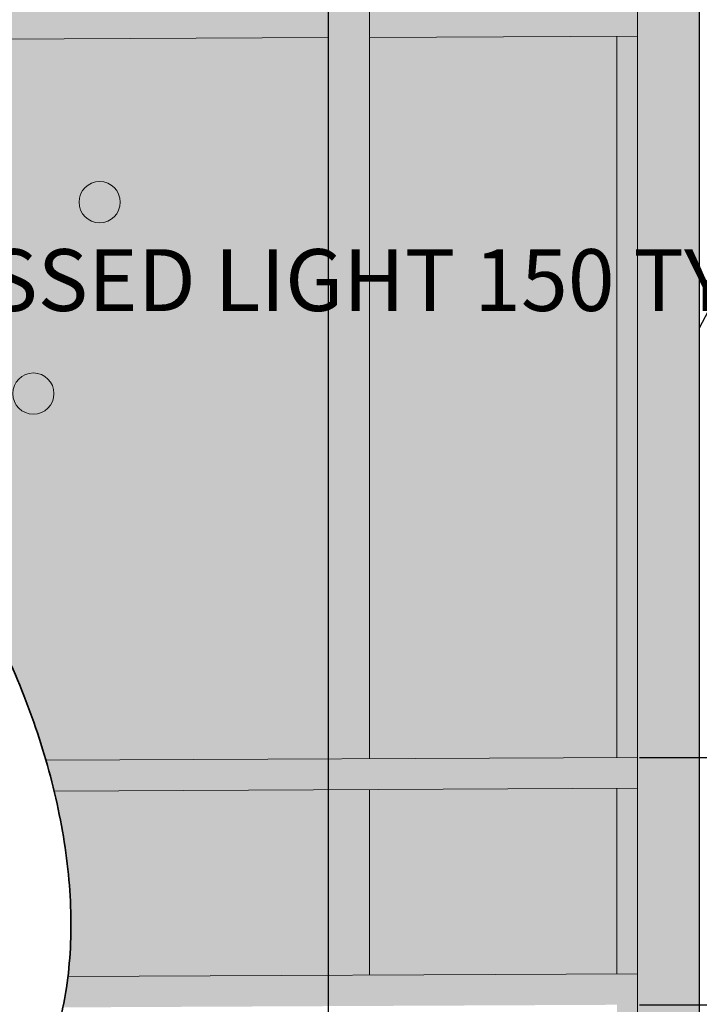
# Model space of a CAD drawing. Units: millimetres. Extents: x 11032 to 26788, y 3406 to 24505.
# Tile 71 of 78: x 21249 to 22897, y 12721 to 15110. Entities that reach past the tile are written whole.
import ezdxf

# ---------------------------------------------------------------- set-up
doc = ezdxf.new("R2010")
doc.units = ezdxf.units.MM
doc.header["$MEASUREMENT"] = 0
for name, color, linetype, lineweight in [('A-ANNO-DIMS', 2, 'Continuous', 18), ('A-GLAZ', 250, 'Continuous', 20), ('A-GLAZ-PATT', 9, 'Continuous', 13), ('A-ROOF', 7, 'Continuous', 30), ('A-WALL', 7, 'Continuous', 35), ('E-LITE', 7, 'Continuous', 18), ('E-LITE-PATT', 7, 'Continuous', 13)]:
    doc.layers.add(name, color=color, linetype=linetype, lineweight=lineweight)
doc.layers.add('A-GLAZ-FRAM-PATT', color=250, linetype='Continuous', lineweight=13, true_color=0x262627)
doc.styles.get("Standard").update_dxf_attribs({"font": 'arial.ttf'})
doc.dimstyles.get("Standard").update_dxf_attribs({"dimtxt": 150, "dimasz": 100, "dimexe": 10, "dimexo": 5, "dimgap": 5, "dimtad": 0, "dimtih": 1, "dimtoh": 1, "dimdec": 0, "dimzin": 0, "dimdsep": 46, "dimtxsty": 'Standard', "dimcen": 0.09, "dimadec": 0, "dimazin": 0, "dimtfac": 1, "dimtdec": 0, "dimtofl": 0, "dimtmove": 0, "dimatfit": 3, "dimfxl": 1, "dimtolj": 1, "dimtzin": 0, "dimarcsym": 0})

# ---------------------------------------------------------------- blocks, each defined once
blk = doc.blocks.new('RECESSED-LIGHT-100')
blk.add_circle((50, 50), 50)
blk = doc.blocks.new('*D20')
at = {"layer": 'A-ANNO-DIMS', "color": 0, "lineweight": -2, "transparency": 16777216}
for p, q in [((21468.9, 12413.4), (21368.9, 12413.4)), ((21568.9, 12403.4), (21568.9, 12423.4)), ((21668.9, 12403.4), (21668.9, 12423.4)), ((21768.9, 12413.4), (21868.9, 12413.4))]:
    blk.add_line(p, q, dxfattribs=at)
at = {"layer": 'A-ANNO-DIMS', "color": 0, "transparency": 16777216}
for points in [[(21468.9, 12430), (21468.9, 12396.7), (21568.9, 12413.4)], [(21768.9, 12430), (21768.9, 12396.7), (21668.9, 12413.4)]]:
    blk.add_solid(points, dxfattribs=at)
at = {"layer": 'Defpoints', "color": 0, "transparency": 16777216}
for p in [(21668.9, 12413.4), (21568.9, 12398.4), (21668.9, 12398.4)]:
    blk.add_point(p, dxfattribs=at)
at = {"layer": 'A-ANNO-DIMS', "color": 0, "transparency": 16777216, "insert": (23236.5, 12413.4), "char_height": 150, "attachment_point": 5}
blk.add_mtext('\\A1;RECESSED LIGHT 100 TYP.', dxfattribs=at)
blk = doc.blocks.new('*D21')
at = {"layer": 'A-ANNO-DIMS', "color": 0, "lineweight": -2, "transparency": 16777216}
for p, q in [((21553.9, 12498.4), (21553.9, 12598.4)), ((21553.9, 12598.4), (21653.9, 12598.4)), ((21563.9, 12398.4), (21543.9, 12398.4)), ((21563.9, 12298.4), (21543.9, 12298.4)), ((21553.9, 12198.4), (21553.9, 12098.4))]:
    blk.add_line(p, q, dxfattribs=at)
at = {"layer": 'A-ANNO-DIMS', "color": 0, "transparency": 16777216}
for points in [[(21537.2, 12498.4), (21570.6, 12498.4), (21553.9, 12398.4)], [(21537.2, 12198.4), (21570.6, 12198.4), (21553.9, 12298.4)]]:
    blk.add_solid(points, dxfattribs=at)
at = {"layer": 'Defpoints', "color": 0, "transparency": 16777216}
for p in [(21553.9, 12398.4), (21568.9, 12398.4), (21568.9, 12298.4)]:
    blk.add_point(p, dxfattribs=at)
at = {"layer": 'A-ANNO-DIMS', "color": 0, "transparency": 16777216, "insert": (22075.2, 12598.4), "char_height": 150, "attachment_point": 5}
blk.add_mtext('\\A1;100 TYP.', dxfattribs=at)
blk = doc.blocks.new('*D22')
at = {"layer": 'A-ANNO-DIMS', "color": 0, "lineweight": -2, "transparency": 16777216}
for p, q in [((20094.7, 14478.3), (19994.7, 14478.3)), ((20194.7, 14460.8), (20194.7, 14488.3)), ((20344.7, 14460.8), (20344.7, 14488.3)), ((20444.7, 14478.3), (20544.7, 14478.3))]:
    blk.add_line(p, q, dxfattribs=at)
at = {"layer": 'A-ANNO-DIMS', "color": 0, "transparency": 16777216}
for points in [[(20094.7, 14495), (20094.7, 14461.7), (20194.7, 14478.3)], [(20444.7, 14495), (20444.7, 14461.7), (20344.7, 14478.3)]]:
    blk.add_solid(points, dxfattribs=at)
at = {"layer": 'Defpoints', "color": 0, "transparency": 16777216}
for p in [(20344.7, 14478.3), (20194.7, 14455.8), (20344.7, 14455.8)]:
    blk.add_point(p, dxfattribs=at)
at = {"layer": 'A-ANNO-DIMS', "color": 0, "transparency": 16777216, "insert": (21912.3, 14478.3), "char_height": 150, "attachment_point": 5}
blk.add_mtext('\\A1;RECESSED LIGHT 150 TYP.', dxfattribs=at)
blk = doc.blocks.new('*D36')
at = {"layer": 'A-ANNO-DIMS', "color": 0, "lineweight": -2, "transparency": 16777216}
for p, q in [((12301.3, 17115.9), (12301.3, 24416.9)), ((12401.3, 24406.9), (18569.2, 24406.9)), ((25297.4, 24406.9), (19129.5, 24406.9)), ((25397.4, 4466.4), (25397.4, 24416.9))]:
    blk.add_line(p, q, dxfattribs=at)
at = {"layer": 'A-ANNO-DIMS', "color": 0, "transparency": 16777216}
for points in [[(12401.3, 24423.5), (12401.3, 24390.2), (12301.3, 24406.9)], [(25297.4, 24423.5), (25297.4, 24390.2), (25397.4, 24406.9)]]:
    blk.add_solid(points, dxfattribs=at)
at = {"layer": 'Defpoints', "color": 0, "transparency": 16777216}
for p in [(25397.4, 24406.9), (12301.3, 17110.9), (25397.4, 4461.4)]:
    blk.add_point(p, dxfattribs=at)
at = {"layer": 'A-ANNO-DIMS', "color": 0, "transparency": 16777216, "insert": (18849.3, 24406.9), "char_height": 150, "attachment_point": 5}
blk.add_mtext('\\A1;13096', dxfattribs=at)
blk = doc.blocks.new('*D42')
at = {"layer": 'A-ANNO-DIMS', "color": 0, "lineweight": -2, "transparency": 16777216}
for p, q in [((22752.4, 13320.1), (26363.9, 13320.1)), ((26353.9, 13220.1), (26353.9, 13101.7)), ((26353.9, 12820.1), (26353.9, 12938.5)), ((22752.4, 12720.1), (26363.9, 12720.1))]:
    blk.add_line(p, q, dxfattribs=at)
at = {"layer": 'A-ANNO-DIMS', "color": 0, "transparency": 16777216}
for points in [[(26337.2, 13220.1), (26370.6, 13220.1), (26353.9, 13320.1)], [(26337.2, 12820.1), (26370.6, 12820.1), (26353.9, 12720.1)]]:
    blk.add_solid(points, dxfattribs=at)
at = {"layer": 'Defpoints', "color": 0, "transparency": 16777216}
for p in [(22747.4, 13320.1), (26353.9, 13320.1), (22747.4, 12720.1)]:
    blk.add_point(p, dxfattribs=at)
at = {"layer": 'A-ANNO-DIMS', "color": 0, "transparency": 16777216, "insert": (26353.9, 13020.1), "char_height": 150, "attachment_point": 5}
blk.add_mtext('\\A1;600', dxfattribs=at)
blk = doc.blocks.new('*D43')
at = {"layer": 'A-ANNO-DIMS', "color": 0, "lineweight": -2, "transparency": 16777216}
for p, q in [((22752.4, 15170.1), (26363.9, 15170.1)), ((26353.9, 15070.1), (26353.9, 14326.7)), ((26353.9, 13420.1), (26353.9, 14163.5)), ((22752.4, 13320.1), (26363.9, 13320.1))]:
    blk.add_line(p, q, dxfattribs=at)
at = {"layer": 'A-ANNO-DIMS', "color": 0, "transparency": 16777216}
for points in [[(26337.2, 15070.1), (26370.6, 15070.1), (26353.9, 15170.1)], [(26337.2, 13420.1), (26370.6, 13420.1), (26353.9, 13320.1)]]:
    blk.add_solid(points, dxfattribs=at)
at = {"layer": 'Defpoints', "color": 0, "transparency": 16777216}
for p in [(22747.4, 15170.1), (26353.9, 15170.1), (22747.4, 13320.1)]:
    blk.add_point(p, dxfattribs=at)
at = {"layer": 'A-ANNO-DIMS', "color": 0, "transparency": 16777216, "insert": (26353.9, 14245.1), "char_height": 150, "attachment_point": 5}
blk.add_mtext('\\A1;1850', dxfattribs=at)
blk = doc.blocks.new('*D51')
at = {"layer": 'A-ANNO-DIMS', "color": 0, "lineweight": -2, "transparency": 16777216}
for p, q in [((21997.4, 16011.6), (21997.4, 3494.9)), ((19697.4, 16000.7), (19697.4, 3494.9)), ((19797.4, 3504.9), (20617.4, 3504.9)), ((21897.4, 3504.9), (21077.4, 3504.9))]:
    blk.add_line(p, q, dxfattribs=at)
at = {"layer": 'A-ANNO-DIMS', "color": 0, "transparency": 16777216}
for points in [[(19797.4, 3521.6), (19797.4, 3488.2), (19697.4, 3504.9)], [(21897.4, 3521.6), (21897.4, 3488.2), (21997.4, 3504.9)]]:
    blk.add_solid(points, dxfattribs=at)
at = {"layer": 'Defpoints', "color": 0, "transparency": 16777216}
for p in [(21997.4, 16016.6), (19697.4, 16005.7), (21997.4, 3504.9)]:
    blk.add_point(p, dxfattribs=at)
at = {"layer": 'A-ANNO-DIMS', "color": 0, "transparency": 16777216, "insert": (20847.4, 3504.9), "char_height": 150, "attachment_point": 5}
blk.add_mtext('\\A1;2300', dxfattribs=at)
blk = doc.blocks.new('*D52')
at = {"layer": 'A-ANNO-DIMS', "color": 0, "lineweight": -2, "transparency": 16777216}
for p, q in [((22897.4, 16213.4), (22897.4, 3494.9)), ((21997.4, 16011.6), (21997.4, 3494.9)), ((22097.4, 3504.9), (22277, 3504.9)), ((22797.4, 3504.9), (22617.9, 3504.9))]:
    blk.add_line(p, q, dxfattribs=at)
at = {"layer": 'A-ANNO-DIMS', "color": 0, "transparency": 16777216}
for points in [[(22097.4, 3521.6), (22097.4, 3488.2), (21997.4, 3504.9)], [(22797.4, 3521.6), (22797.4, 3488.2), (22897.4, 3504.9)]]:
    blk.add_solid(points, dxfattribs=at)
at = {"layer": 'Defpoints', "color": 0, "transparency": 16777216}
for p in [(22897.4, 16218.4), (21997.4, 16016.6), (22897.4, 3504.9)]:
    blk.add_point(p, dxfattribs=at)
at = {"layer": 'A-ANNO-DIMS', "color": 0, "transparency": 16777216, "insert": (22447.4, 3504.9), "char_height": 150, "attachment_point": 5}
blk.add_mtext('\\A1;900', dxfattribs=at)

msp = doc.modelspace()

# ---------------------------------------------------------------- hatches: boundary and pattern name
at = {"layer": 'A-GLAZ-FRAM-PATT'}
h = msp.add_hatch(color=256, dxfattribs=at)
h.paths.add_polyline_path([(22747.404, 16218.44), (22395.025, 16218.44), (18518.2, 16200.148), (18519.143, 16000.151), (22747.404, 16020.1)])
edge = h.paths.add_edge_path()
edge.add_line((22897.404, 16218.44), (22747.404, 16218.44))
edge.add_line((22747.404, 16218.44), (22747.404, 16020.1))
edge.add_line((22747.404, 16020.1), (22747.404, 9631.346))
edge.add_spline(control_points=[(22747.404, 9631.346), (22803.273, 9520.228), (22853.467, 9405.87), (22897.404, 9289.211)], knot_values=[2645.78092422, 2645.78092422, 2645.78092422, 2645.78092422, 3013.05623672, 3013.05623672, 3013.05623672, 3013.05623672], degree=3, periodic=0)
edge.add_line((22897.404, 9289.211), (22897.404, 16218.44))
h.paths.add_polyline_path([(22097.404, 16017.033), (21997.404, 16016.562), (21997.404, 13316.532), (22097.404, 13317.003)])
edge = h.paths.add_edge_path()
edge.add_line((19797.404, 16006.182), (19697.404, 16005.71))
edge.add_line((19697.404, 16005.71), (19697.404, 15155.703))
edge.add_line((19697.404, 15155.703), (19697.404, 12747.012))
edge.add_spline(control_points=[(19697.404, 12747.012), (19708.389, 12750.081), (19719.253, 12753.406), (19732.457, 12757.789), (19734.918, 12758.62), (19737.372, 12759.464)], knot_values=[1372.60477099, 1372.60477099, 1372.60477099, 1372.60477099, 1399.44343377, 1399.44343377, 1405.61279972, 1405.61279972, 1405.61279972, 1405.61279972], degree=3, periodic=0)
edge.add_spline(control_points=[(19737.372, 12759.464), (19750.245, 12763.891), (19762.932, 12768.657), (19778.9, 12775.14), (19782.354, 12776.572), (19785.794, 12778.028)], knot_values=[1405.61279972, 1405.61279972, 1405.61279972, 1405.61279972, 1437.96891336, 1437.96891336, 1446.94640473, 1446.94640473, 1446.94640473, 1446.94640473], degree=3, periodic=0)
edge.add_spline(control_points=[(19785.794, 12778.028), (19789.682, 12779.673), (19793.552, 12781.348), (19797.404, 12783.051)], knot_values=[1446.94640473, 1446.94640473, 1446.94640473, 1446.94640473, 1457.09545574, 1457.09545574, 1457.09545574, 1457.09545574], degree=3, periodic=0)
edge.add_line((19797.404, 12783.051), (19797.404, 15306.174))
edge.add_line((19797.404, 15306.174), (19797.404, 16006.182))
h = msp.add_hatch(color=256, dxfattribs=at)
h.paths.add_polyline_path([(22747.404, 16020.1), (22697.404, 16019.864), (22697.404, 15169.858), (22747.404, 15170.094)])
h.paths.add_polyline_path([(22747.404, 15070.092), (22697.404, 15069.857), (22697.404, 13319.834), (22747.404, 13320.07)])
edge = h.paths.add_edge_path()
edge.add_line((22747.404, 12795.064), (21365.955, 12788.546))
edge.add_spline(control_points=[(21365.955, 12788.546), (21365.556, 12785.216), (21365.14, 12781.894), (21364.707, 12778.582)], knot_values=[4871.89074498, 4871.89074498, 4871.89074498, 4871.89074498, 4881.51384723, 4881.51384723, 4881.51384723, 4881.51384723], degree=3, periodic=0)
edge.add_spline(control_points=[(21364.707, 12778.582), (21363.953, 12772.805), (21363.147, 12767.057), (21359.867, 12745.141), (21357.035, 12729.186), (21353.796, 12713.488)], knot_values=[4881.51384723, 4881.51384723, 4881.51384723, 4881.51384723, 4898.30109774, 4898.30109774, 4945.85686537, 4945.85686537, 4945.85686537, 4945.85686537], degree=3, periodic=0)
edge.add_line((21353.796, 12713.488), (22747.404, 12720.064))
edge.add_line((22747.404, 12720.064), (22747.404, 12795.064))
edge = h.paths.add_edge_path()
edge.add_line((22747.404, 13320.07), (22697.404, 13319.834))
edge.add_line((22697.404, 13319.834), (21312.567, 13313.3))
edge.add_spline(control_points=[(21312.567, 13313.3), (21312.567, 13313.3), (21312.567, 13313.3), (21312.567, 13313.3)], knot_values=[4405.86932069, 4405.86932069, 4405.86932069, 4405.86932069, 4405.86932536, 4405.86932536, 4405.86932536, 4405.86932536], degree=3, periodic=0)
edge.add_spline(control_points=[(21312.567, 13313.3), (21316.329, 13300.292), (21319.935, 13287.252), (21326.522, 13262.273), (21329.53, 13250.337), (21332.397, 13238.393)], knot_values=[4405.86932536, 4405.86932536, 4405.86932536, 4405.86932536, 4439.73791994, 4439.73791994, 4470.65028407, 4470.65028407, 4470.65028407, 4470.65028407], degree=3, periodic=0)
edge.add_line((21332.397, 13238.393), (22747.404, 13245.069))
edge.add_line((22747.404, 13245.069), (22747.404, 13320.07))
h.paths.add_polyline_path([(22747.404, 13245.069), (22697.404, 13244.833), (22697.404, 12794.828), (22747.404, 12795.064)])
h.paths.add_polyline_path([(22747.404, 12720.064), (22697.404, 12719.828), (22697.404, 11219.811), (22747.404, 11220.047)])
edge = h.paths.add_edge_path()
edge.add_line((22747.404, 11120.046), (22697.404, 11119.81))
edge.add_line((22697.404, 11119.81), (22697.404, 9727.135))
edge.add_spline(control_points=[(22697.404, 9727.135), (22714.538, 9695.493), (22731.209, 9663.555), (22747.404, 9631.346)], knot_values=[2539.32128955, 2539.32128955, 2539.32128955, 2539.32128955, 2645.78092422, 2645.78092422, 2645.78092422, 2645.78092422], degree=3, periodic=0)
edge.add_line((22747.404, 9631.346), (22747.404, 11120.046))
h = msp.add_hatch(color=256, dxfattribs=at)
h.paths.add_polyline_path([(19697.404, 15155.703), (18523.154, 15150.163), (18523.626, 15050.164), (19697.404, 15055.702)])
h.paths.add_polyline_path([(21997.404, 15166.555), (19797.404, 15156.175), (19797.404, 15056.174), (20912.335, 15061.434, -0.11801722), (20947.253, 15061.599), (21997.404, 15066.554)])
h.paths.add_polyline_path([(22747.404, 15170.094), (22097.404, 15167.027), (22097.404, 15067.026), (22747.404, 15070.092)])
edge = h.paths.add_edge_path()
edge.add_line((21997.404, 13241.531), (21332.397, 13238.393))
edge.add_spline(control_points=[(21332.397, 13238.393), (21338.038, 13214.902), (21343.139, 13191.382), (21354.5, 13132.481), (21360.029, 13097.149), (21368.306, 13027.119), (21371.052, 12992.421), (21373.63, 12924.101), (21373.462, 12890.481), (21370.61, 12834.187), (21368.665, 12811.15), (21365.955, 12788.546)], knot_values=[4470.65028407, 4470.65028407, 4470.65028407, 4470.65028407, 4531.4505555, 4531.4505555, 4623.16319106, 4623.16319106, 4714.87582662, 4714.87582662, 4806.58846218, 4806.58846218, 4871.89074498, 4871.89074498, 4871.89074498, 4871.89074498], degree=3, periodic=0)
edge.add_line((21365.955, 12788.546), (21997.404, 12791.526))
edge.add_line((21997.404, 12791.526), (21997.404, 13241.531))
h.paths.add_polyline_path([(22097.404, 13242.003), (21997.404, 13241.531), (21997.404, 12791.526), (22097.404, 12791.998)])
h.paths.add_polyline_path([(22697.404, 13244.833), (22097.404, 13242.003), (22097.404, 12791.998), (22697.404, 12794.828)])
at = {"layer": 'A-GLAZ-PATT'}
h = msp.add_hatch(color=256, dxfattribs=at)
h.set_gradient(color1=(254, 221, 154), color2=(248, 246, 176), name='CURVED')
edge = h.paths.add_edge_path()
edge.add_spline(control_points=[(18522.918, 15200.175), (18561.599, 15201.209), (18600.224, 15202.243), (18716.594, 15205.749), (18794.099, 15208.613), (18948.086, 15217.451), (19024.568, 15223.425), (19176.135, 15240.511), (19251.219, 15251.623), (19333.848, 15267.966), (19342.25, 15269.676), (19356.967, 15272.758), (19363.289, 15274.111), (19375.94, 15276.871), (19382.267, 15278.279), (19401.252, 15282.576), (19413.915, 15285.541), (19451.935, 15294.685), (19477.322, 15301.111), (19548.254, 15319.552), (19593.948, 15331.984), (19659.079, 15349.253), (19678.203, 15354.269), (19697.404, 15359.188)], knot_values=[1.09285599, 1.09285599, 1.09285599, 1.09285599, 116.34451384, 116.34451384, 349.03354152, 349.03354152, 581.72256921, 581.72256921, 814.41159689, 814.41159689, 840.78637359, 840.78637359, 860.67891922, 860.67891922, 880.57146485, 880.57146485, 920.35655611, 920.35655611, 999.92673863, 999.92673863, 1142.09604805, 1142.09604805, 1200.90860694, 1200.90860694, 1200.90860694, 1200.90860694], degree=3, periodic=0)
edge.add_line((19697.404, 15359.188), (19697.404, 16005.71))
edge.add_line((19697.404, 16005.71), (18519.143, 16000.151))
edge.add_line((18519.143, 16000.151), (18522.918, 15200.175))
edge = h.paths.add_edge_path()
edge.add_line((19697.404, 15055.702), (18523.626, 15050.164))
edge.add_line((18523.626, 15050.164), (18531.851, 13306.733))
edge.add_spline(control_points=[(18531.851, 13306.733), (18553.325, 13284.933), (18574.901, 13263.301), (18632.771, 13206.214), (18669.261, 13171.188), (18735.852, 13109.762), (18765.813, 13083.011), (18826.398, 13031.156), (18857.021, 13006.052), (18919.15, 12957.862), (18950.655, 12934.774), (19007.615, 12895.967), (19032.834, 12879.759), (19084.165, 12849.05), (19110.278, 12834.547), (19163.6, 12807.555), (19190.811, 12795.065), (19240.068, 12775.123), (19261.85, 12767.175), (19306.233, 12752.949), (19328.834, 12746.672), (19374.859, 12736.071), (19398.283, 12731.748), (19445.866, 12725.365), (19470.026, 12723.306), (19514.597, 12721.889), (19534.921, 12722.121), (19575.756, 12724.466), (19596.267, 12726.579), (19622.683, 12730.57), (19628.6, 12731.546), (19638.601, 12733.337), (19642.688, 12734.108), (19650.826, 12735.723), (19654.881, 12736.567), (19667.001, 12739.207), (19675.023, 12741.111), (19687.813, 12744.388), (19692.62, 12745.676), (19697.404, 12747.012)], knot_values=[259.28299856, 259.28299856, 259.28299856, 259.28299856, 332.45020059, 332.45020059, 454.53383699, 454.53383699, 552.84889009, 552.84889009, 651.16394319, 651.16394319, 749.47899629, 749.47899629, 825.6298474, 825.6298474, 901.7806985, 901.7806985, 977.9315496, 977.9315496, 1036.43952646, 1036.43952646, 1094.94750331, 1094.94750331, 1153.45548017, 1153.45548017, 1211.96345702, 1211.96345702, 1260.21270617, 1260.21270617, 1308.46195531, 1308.46195531, 1322.39247458, 1322.39247458, 1332.02384448, 1332.02384448, 1341.65521438, 1341.65521438, 1360.91795418, 1360.91795418, 1372.60477099, 1372.60477099, 1372.60477099, 1372.60477099], degree=3, periodic=0)
edge.add_line((19697.404, 12747.012), (19697.404, 15055.702))
h.paths.add_polyline_path([(18790.086, 14298.34, -1), (18890.086, 14298.34, -1)], flags=16)
h.paths.add_polyline_path([(19437.524, 14550.125, -1), (19537.524, 14550.125, -1)], flags=16)
h.paths.add_polyline_path([(22697.404, 16019.864), (22097.404, 16017.033), (22097.404, 15167.027), (22697.404, 15169.858)])
h.paths.add_polyline_path([(22697.404, 15069.857), (22097.404, 15067.026), (22097.404, 13317.003), (22697.404, 13319.834)])
h.paths.add_polyline_path([(20866.429, 15795.606, -1), (21016.429, 15795.606, -1)], flags=16)
h.paths.add_polyline_path([(19822.441, 15337.78), (19797.404, 15332.147), (19797.404, 15156.175), (20721.869, 15160.537), (20700.803, 15175.665), (20679.512, 15190.548), (20657.993, 15205.143), (20636.247, 15219.41), (20614.273, 15233.307), (20592.07, 15246.794), (20569.639, 15259.829), (20546.978, 15272.372), (20524.088, 15284.38), (20500.968, 15295.814), (20477.616, 15306.631), (20454.034, 15316.792), (20430.219, 15326.254), (20406.173, 15334.976), (20381.894, 15342.919), (20357.382, 15350.039), (20332.636, 15356.297), (20307.662, 15361.667), (20282.483, 15366.173), (20257.125, 15369.849), (20231.617, 15372.729), (20205.984, 15374.847), (20180.253, 15376.236), (20154.451, 15376.931), (20128.605, 15376.964), (20102.742, 15376.37), (20076.889, 15375.183), (20051.072, 15373.436), (20025.318, 15371.163), (19999.653, 15368.398), (19974.087, 15365.173), (19948.614, 15361.516), (19923.228, 15357.456), (19897.924, 15353.024), (19872.695, 15348.248), (19847.536, 15343.157)])
h.paths.add_polyline_path([(19797.404, 15383.428), (19822.666, 15388.998), (19848.044, 15394.311), (19873.542, 15399.338), (19899.168, 15404.048), (19924.927, 15408.41), (19950.824, 15412.396), (19976.865, 15415.972), (20003.054, 15419.109), (20029.394, 15421.774), (20055.871, 15423.934), (20082.461, 15425.553), (20109.142, 15426.594), (20135.888, 15427.02), (20162.676, 15426.794), (20189.481, 15425.88), (20216.28, 15424.237), (20243.046, 15421.828), (20269.754, 15418.614), (20296.377, 15414.554), (20322.887, 15409.61), (20349.254, 15403.74), (20375.368, 15396.947), (20401.163, 15389.283), (20426.64, 15380.795), (20451.799, 15371.531), (20476.643, 15361.538), (20501.172, 15350.863), (20525.391, 15339.55), (20549.302, 15327.645), (20572.91, 15315.192), (20596.218, 15302.234), (20619.229, 15288.816), (20641.948, 15274.978), (20664.378, 15260.764), (20686.523, 15246.215), (20708.386, 15231.373), (20729.97, 15216.279), (20751.277, 15200.974), (20806.33, 15160.935), (21997.404, 15166.555), (21997.404, 16016.562), (19797.404, 16006.182)])
h = msp.add_hatch(color=256, dxfattribs=at)
h.set_gradient(color1=(254, 221, 154), color2=(248, 246, 176), name='CURVED')
edge = h.paths.add_edge_path()
edge.add_spline(control_points=[(19797.404, 12783.051), (19804.766, 12786.308), (19812.062, 12789.67), (19840.433, 12803.253), (19861.01, 12814.224), (19901.109, 12837.623), (19920.632, 12850.05), (19958.72, 12876.17), (19977.285, 12889.863), (20013.556, 12918.366), (20031.262, 12933.177), (20065.902, 12963.799), (20082.836, 12979.61), (20116.005, 13012.138), (20132.242, 13028.855), (20172.106, 13071.751), (20195.333, 13098.449), (20240.492, 13153.453), (20262.424, 13181.759), (20305.087, 13239.746), (20325.817, 13269.427), (20366.129, 13329.934), (20385.709, 13360.76), (20423.742, 13423.329), (20442.194, 13455.072), (20468.125, 13501.581), (20476.052, 13516.073), (20488.875, 13539.954), (20493.837, 13549.308), (20502.675, 13566.165), (20506.568, 13573.661), (20512.937, 13586.042), (20515.432, 13590.92), (20520.037, 13599.983), (20522.152, 13604.167), (20526.352, 13612.516), (20528.438, 13616.684), (20534.656, 13629.168), (20538.749, 13637.462), (20550.88, 13662.246), (20558.771, 13678.635), (20578.692, 13720.455), (20590.467, 13745.616), (20613.331, 13794.631), (20624.42, 13818.484), (20646.021, 13864.438), (20656.535, 13886.538), (20675.091, 13924.525), (20683.225, 13940.795), (20699.114, 13971.559), (20706.87, 13986.053), (20721.908, 14012.944), (20729.192, 14025.339), (20741.464, 14045.078), (20746.591, 14052.924), (20756.302, 14067.035), (20760.886, 14073.298), (20769.297, 14084.118), (20773.125, 14088.673), (20778.393, 14094.528), (20780.172, 14096.399), (20781.73, 14097.965)], knot_values=[1457.09545574, 1457.09545574, 1457.09545574, 1457.09545574, 1476.49439296, 1476.49439296, 1533.22155094, 1533.22155094, 1589.94870892, 1589.94870892, 1646.6758669, 1646.6758669, 1703.40302488, 1703.40302488, 1760.13018286, 1760.13018286, 1816.85734084, 1816.85734084, 1902.20435658, 1902.20435658, 1987.55137233, 1987.55137233, 2072.89838807, 2072.89838807, 2158.24540381, 2158.24540381, 2243.59241956, 2243.59241956, 2281.95910756, 2281.95910756, 2306.55775766, 2306.55775766, 2326.19089392, 2326.19089392, 2338.93304435, 2338.93304435, 2349.84264561, 2349.84264561, 2360.75224686, 2360.75224686, 2382.57144936, 2382.57144936, 2426.20985437, 2426.20985437, 2495.17510968, 2495.17510968, 2564.14036499, 2564.14036499, 2633.1056203, 2633.1056203, 2689.03366063, 2689.03366063, 2744.96170095, 2744.96170095, 2800.88974128, 2800.88974128, 2843.74245207, 2843.74245207, 2886.59516287, 2886.59516287, 2929.44787366, 2929.44787366, 2954.91871542, 2954.91871542, 2954.91871542, 2954.91871542], degree=3, periodic=0)
edge.add_spline(control_points=[(20781.73, 14097.965), (20784.285, 14097.292), (20787.436, 14096.331), (20794.831, 14093.655), (20799.074, 14091.941), (20808.517, 14087.64), (20813.716, 14085.055), (20824.925, 14078.948), (20830.934, 14075.426), (20843.621, 14067.418), (20850.299, 14062.932), (20864.197, 14052.997), (20871.416, 14047.547), (20889.597, 14033.059), (20900.79, 14023.505), (20923.774, 14002.511), (20935.566, 13991.072), (20959.505, 13966.429), (20971.653, 13953.226), (20996.104, 13925.188), (21008.407, 13910.354), (21032.993, 13879.192), (21045.278, 13862.864), (21075.715, 13820.438), (21093.762, 13793.504), (21129.039, 13737.067), (21146.269, 13707.566), (21179.532, 13646.451), (21195.565, 13614.838), (21226.093, 13549.956), (21240.587, 13516.686), (21267.729, 13448.943), (21280.375, 13414.47), (21299.261, 13357.645), (21306.142, 13335.518), (21312.567, 13313.3)], knot_values=[3328.11564031, 3328.11564031, 3328.11564031, 3328.11564031, 3370.54654151, 3370.54654151, 3412.97744272, 3412.97744272, 3455.40834392, 3455.40834392, 3497.83924512, 3497.83924512, 3540.27014632, 3540.27014632, 3582.70104752, 3582.70104752, 3644.05325934, 3644.05325934, 3705.40547115, 3705.40547115, 3766.75768296, 3766.75768296, 3828.10989477, 3828.10989477, 3889.46210658, 3889.46210658, 3981.17474214, 3981.17474214, 4072.8873777, 4072.8873777, 4164.60001326, 4164.60001326, 4256.31264882, 4256.31264882, 4348.02528438, 4348.02528438, 4405.86932069, 4405.86932069, 4405.86932069, 4405.86932069], degree=3, periodic=0)
edge.add_line((21312.567, 13313.3), (21997.404, 13316.532))
edge.add_line((21997.404, 13316.532), (21997.404, 15066.554))
edge.add_line((21997.404, 15066.554), (20947.253, 15061.599))
edge.add_arc((20930.138, 14988.578), 75, 0, 76.808818, ccw=False)
edge.add_arc((20930.138, 14988.578), 75, -180, 0, ccw=False)
edge.add_arc((20930.138, 14988.578), 75, 103.731838, 180, ccw=False)
edge.add_line((20912.335, 15061.434), (19797.404, 15056.174))
edge.add_line((19797.404, 15056.174), (19797.404, 12783.051))
h.paths.add_polyline_path([(20194.664, 14380.821, -1), (20344.664, 14380.821, -1)], flags=16)
h.paths.add_polyline_path([(20594.425, 14224.541, -1), (20744.425, 14224.541, -1)], flags=16)
h.paths.add_polyline_path([(19868.772, 14780.204, -1), (20018.772, 14780.204, -1)], flags=16)
h.paths.add_polyline_path([(20754.127, 14602.218, -1), (20854.127, 14602.218, -1)], flags=16)
h.paths.add_polyline_path([(21232.101, 14202.835, -1), (21332.101, 14202.835, -1)], flags=16)
h.paths.add_polyline_path([(21392.875, 14667.335, -1), (21492.875, 14667.335, -1)], flags=16)
at = {"layer": 'E-LITE-PATT'}
h = msp.add_hatch(color=256, dxfattribs=at)
h.paths.add_polyline_path([(23729.349, 12537.488, 1), (23529.349, 12537.488, 1)])
h.paths.add_polyline_path([(24163.611, 13699.89, 1), (23963.611, 13699.89, 1)])
h.paths.add_polyline_path([(18790.086, 14298.34, 1), (18890.086, 14298.34, 1)])
h.paths.add_polyline_path([(19537.524, 14550.125, 1), (19437.524, 14550.125, 1)])
h.paths.add_polyline_path([(20194.664, 14380.821, 1), (20344.664, 14380.821, 1)])
h.paths.add_polyline_path([(20018.772, 14780.204, 1), (19868.772, 14780.204, 1)])
h.paths.add_polyline_path([(20594.425, 14224.541, 1), (20744.425, 14224.541, 1)])
h.paths.add_polyline_path([(21232.101, 14202.835, 1), (21332.101, 14202.835, 1)])
h.paths.add_polyline_path([(20854.127, 14602.218, 1), (20754.127, 14602.218, 1)])
h.paths.add_polyline_path([(21492.875, 14667.335, 1), (21392.875, 14667.335, 1)])
h.paths.add_polyline_path([(21005.138, 14988.578, 1), (20855.138, 14988.578, 1)])
h = msp.add_hatch(color=256, dxfattribs=at)
h.paths.add_polyline_path([(21120.849, 11395.371, 1), (21220.849, 11395.371, 1)])
h.paths.add_polyline_path([(21215.053, 11595.746, 1), (21315.053, 11595.746, 1)])
h.paths.add_polyline_path([(21407.506, 11792.395, 1), (21307.506, 11792.395, 1)])
h.paths.add_polyline_path([(21507.11, 12004.255, 1), (21407.11, 12004.255, 1)])
h.paths.add_polyline_path([(21501.367, 12204.741, 1), (21601.367, 12204.741, 1)])
h.paths.add_polyline_path([(21668.897, 12348.379, 1), (21568.897, 12348.379, 1)])
h.paths.add_polyline_path([(23729.349, 12537.488, 1), (23529.349, 12537.488, 1)])
h.paths.add_polyline_path([(23963.611, 13699.89, 1), (24163.611, 13699.89, 1)])
h.paths.add_polyline_path([(21492.875, 14667.335, 1), (21392.875, 14667.335, 1)])
h.paths.add_polyline_path([(21332.101, 14202.835, 1), (21232.101, 14202.835, 1)])
h.paths.add_polyline_path([(20744.425, 14224.541, 1), (20594.425, 14224.541, 1)])
h.paths.add_polyline_path([(20854.127, 14602.218, 1), (20754.127, 14602.218, 1)])
h.paths.add_polyline_path([(20947.253, 15061.599), (20912.335, 15061.434, 0.34563694), (20855.138, 14988.578, 1), (21005.138, 14988.578, 0.34827999)])

# ---------------------------------------------------------------- linework, layer by layer
at = {"layer": 'A-GLAZ'}
for p, q in [((22747.404, 16218.44), (22747.404, 9631.346)), ((21997.404, 16016.562), (21997.404, 13316.532)), ((22097.404, 16017.033), (22097.404, 13317.003)), ((21997.404, 15066.554), (19797.404, 15056.174)), ((22747.404, 15070.092), (22097.404, 15067.026)), ((22697.404, 15069.857), (22697.404, 13319.834)), ((22747.404, 13320.07), (21312.567, 13313.3)), ((22747.404, 13245.069), (21332.397, 13238.393)), ((21997.404, 13241.531), (21997.404, 12791.526)), ((22097.404, 13242.003), (22097.404, 12791.998)), ((22697.404, 13244.833), (22697.404, 12794.828)), ((22747.404, 12795.064), (21365.955, 12788.546))]:
    msp.add_line(p, q, dxfattribs=at)
at = {"layer": 'A-ROOF'}
msp.add_open_spline([(19305.291, 17259.568), (19382.851, 17264.718), (19460.41, 17269.868), (19537.97, 17275.018), (19654.15, 17282.732), (19770.33, 17290.447), (19886.51, 17298.161), (19886.51, 17298.161), (19886.51, 17298.161), (19886.51, 17298.161), (20092.886, 17311.864), (21679.83, 17482.933), (25498.5, 17958.124), (23655.645, 15804.534), (22897.404, 14361.22)], degree=3, knots=[8878.9087223, 8878.9087223, 8878.9087223, 8878.9087223, 9101.65833771, 9101.65833771, 9101.65833771, 9435.32303857, 9435.32303857, 9435.32303857, 9435.32329041, 9435.32329041, 9435.32329041, 10028.02667108, 13760.8945204, 16370.50452639, 16370.50452639, 16370.50452639, 16370.50452639], dxfattribs=at)
at = {"layer": 'A-WALL'}
msp.add_open_spline([(20781.73, 14097.965), (20784.285, 14097.292), (20787.436, 14096.331), (20794.831, 14093.655), (20799.074, 14091.941), (20808.517, 14087.64), (20813.716, 14085.055), (20824.925, 14078.948), (20830.934, 14075.426), (20843.621, 14067.418), (20850.299, 14062.932), (20864.197, 14052.997), (20871.416, 14047.547), (20889.597, 14033.059), (20900.79, 14023.505), (20923.774, 14002.511), (20935.566, 13991.072), (20959.505, 13966.429), (20971.653, 13953.226), (20996.104, 13925.188), (21008.407, 13910.354), (21032.993, 13879.192), (21045.278, 13862.864), (21075.715, 13820.438), (21093.762, 13793.504), (21129.039, 13737.067), (21146.269, 13707.566), (21179.532, 13646.451), (21195.565, 13614.838), (21226.093, 13549.956), (21240.587, 13516.686), (21267.729, 13448.943), (21280.375, 13414.47), (21303.538, 13344.776), (21314.054, 13309.556), (21332.704, 13238.828), (21340.837, 13203.321), (21354.5, 13132.481), (21360.029, 13097.149), (21368.306, 13027.119), (21371.052, 12992.421), (21373.63, 12924.101), (21373.462, 12890.481), (21370.13, 12824.718), (21366.968, 12792.577), (21358.463, 12735.763), (21353.621, 12710.793), (21345.944, 12678.95), (21344.029, 12671.478), (21341.252, 12661.256), (21340.473, 12658.452), (21338.881, 12652.839), (21338.068, 12650.032), (21335.58, 12641.609), (21333.854, 12635.993), (21328.479, 12619.14), (21324.632, 12607.899), (21312.219, 12573.877), (21302.855, 12551.077), (21282.165, 12505.474), (21270.839, 12482.672), (21246.416, 12437.152), (21233.319, 12414.435), (21205.588, 12369.182), (21190.953, 12346.647), (21160.407, 12301.852), (21144.496, 12279.592), (21111.679, 12235.428), (21094.773, 12213.524), (21055.718, 12164.423), (21033.359, 12137.352), (20988.115, 12083.954), (20965.231, 12057.628), (20919.516, 12005.731), (20896.686, 11980.16), (20857.367, 11936.124), (20840.745, 11917.509), (20808.035, 11880.563), (20791.947, 11862.233), (20763.475, 11829.178), (20750.967, 11814.43), (20726.5, 11784.882), (20714.539, 11770.084), (20693.385, 11742.981), (20684.087, 11730.721), (20665.941, 11705.856), (20657.092, 11693.252), (20641.315, 11669.592), (20634.312, 11658.625), (20620.703, 11636.087), (20614.097, 11624.517), (20601.376, 11600.52), (20595.259, 11588.093), (20585.03, 11565.079), (20580.781, 11554.73), (20572.815, 11533.181), (20569.097, 11521.98), (20562.398, 11498.577), (20559.418, 11486.373), (20555.045, 11463.74), (20553.448, 11453.531), (20551.046, 11432.459), (20550.243, 11421.596), (20549.62, 11399.291), (20549.802, 11387.848), (20551.33, 11364.54), (20552.678, 11352.676), (20556.671, 11328.775), (20559.317, 11316.74), (20565.954, 11292.813), (20569.944, 11280.922), (20579.202, 11257.616), (20584.469, 11246.202), (20592.114, 11231.712), (20593.991, 11228.293), (20597.158, 11222.745), (20598.418, 11220.59), (20600.975, 11216.322), (20602.269, 11214.214), (20606.192, 11207.964), (20608.863, 11203.899), (20617.481, 11191.329), (20623.597, 11183.201), (20636.089, 11167.852), (20642.464, 11160.629), (20655.347, 11147.002), (20661.856, 11140.596), (20674.924, 11128.498), (20681.484, 11122.806), (20694.608, 11112.032), (20701.171, 11106.95), (20714.277, 11097.303), (20720.82, 11092.738), (20737.095, 11081.899), (20746.81, 11075.891), (20766.189, 11064.614), (20775.854, 11059.347), (20795.171, 11049.382), (20804.823, 11044.686), (20824.152, 11035.736), (20833.829, 11031.484), (20853.244, 11023.327), (20862.982, 11019.423), (20887.017, 11010.17), (20901.366, 11004.975), (20930.315, 10995.005), (20944.916, 10990.23), (20967.117, 10983.27), (20974.61, 10980.971), (20982.141, 10978.705), (20982.141, 10978.705), (20982.141, 10978.705), (20982.141, 10978.705), (21260.768, 10894.876), (21539.396, 10811.046), (21803.195, 10686.28), (21811.686, 10678.824), (21810.573, 10681.187), (21811.406, 10681.686), (21870.06, 10660.606), (21925.845, 10628.283), (21978.958, 10591.693)], degree=3, knots=[3328.11564031, 3328.11564031, 3328.11564031, 3328.11564031, 3370.54654151, 3370.54654151, 3412.97744272, 3412.97744272, 3455.40834392, 3455.40834392, 3497.83924512, 3497.83924512, 3540.27014632, 3540.27014632, 3582.70104752, 3582.70104752, 3644.05325934, 3644.05325934, 3705.40547115, 3705.40547115, 3766.75768296, 3766.75768296, 3828.10989477, 3828.10989477, 3889.46210658, 3889.46210658, 3981.17474214, 3981.17474214, 4072.8873777, 4072.8873777, 4164.60001326, 4164.60001326, 4256.31264882, 4256.31264882, 4348.02528438, 4348.02528438, 4439.73791994, 4439.73791994, 4531.4505555, 4531.4505555, 4623.16319106, 4623.16319106, 4714.87582662, 4714.87582662, 4806.58846218, 4806.58846218, 4898.30109774, 4898.30109774, 4973.3893459, 4973.3893459, 4996.66899489, 4996.66899489, 5005.51338613, 5005.51338613, 5014.35777737, 5014.35777737, 5032.04655985, 5032.04655985, 5067.42412481, 5067.42412481, 5139.05868364, 5139.05868364, 5210.69324248, 5210.69324248, 5282.32780131, 5282.32780131, 5353.96236015, 5353.96236015, 5425.59691898, 5425.59691898, 5497.23147782, 5497.23147782, 5587.7210555, 5587.7210555, 5678.21063318, 5678.21063318, 5768.70021086, 5768.70021086, 5836.11850381, 5836.11850381, 5903.53679676, 5903.53679676, 5958.13178915, 5958.13178915, 6012.72678154, 6012.72678154, 6057.24703228, 6057.24703228, 6101.76728303, 6101.76728303, 6138.92040589, 6138.92040589, 6176.07352875, 6176.07352875, 6213.2266516, 6213.2266516, 6241.78247951, 6241.78247951, 6270.33830742, 6270.33830742, 6298.89413533, 6298.89413533, 6321.01839771, 6321.01839771, 6343.1426601, 6343.1426601, 6365.26692248, 6365.26692248, 6387.39118486, 6387.39118486, 6409.51544725, 6409.51544725, 6431.63970963, 6431.63970963, 6453.76397201, 6453.76397201, 6460.69362746, 6460.69362746, 6465.1443277, 6465.1443277, 6469.59502793, 6469.59502793, 6478.49642841, 6478.49642841, 6497.82694928, 6497.82694928, 6517.15747016, 6517.15747016, 6536.48799103, 6536.48799103, 6555.81851191, 6555.81851191, 6575.14903278, 6575.14903278, 6594.47955366, 6594.47955366, 6623.33387959, 6623.33387959, 6652.18820553, 6652.18820553, 6681.04253146, 6681.04253146, 6709.89685739, 6709.89685739, 6738.75118333, 6738.75118333, 6780.7900818, 6780.7900818, 6822.82898026, 6822.82898026, 6844.09412613, 6844.09412613, 6844.09412613, 6844.09478462, 6844.09478462, 6844.09478462, 7630.91131707, 7630.91131707, 7630.91131707, 7630.91175685, 7630.91175685, 7630.91175685, 7795.92722484, 7795.92722484, 7795.92722484, 7795.92722484], dxfattribs=at)

# ---------------------------------------------------------------- block references
at = {"layer": 'E-LITE'}
for p in [(21392.875, 14617.335), (21232.102, 14152.835)]:
    msp.add_blockref('RECESSED-LIGHT-100', p, dxfattribs=at)

# ---------------------------------------------------------------- dimensions: what is measured, and where the dimension line sits
at = {"layer": 'A-ANNO-DIMS'}
for base, p1, p2, picture, middle in [((25397.404, 24406.858), (12301.265, 17110.885), (25397.404, 4461.399), '*D36', (18849.334, 24406.858)), ((22897.404, 3504.899), (21997.404, 16016.562), (22897.404, 16218.44), '*D52', (22447.404, 3504.899)), ((21997.404, 3504.899), (19697.404, 16005.71), (21997.404, 16016.562), '*D51', (20847.404, 3504.899))]:
    dim = msp.add_linear_dim(base=base, p1=p1, p2=p2, dimstyle='Standard', override={"dimdec": 0, "dimlfac": 1, "dimrnd": 0, "dimzin": 0, "dimdsep": 46, "dimlunit": 2}, dxfattribs=at)
    dim.commit()
    dim.dimension.update_dxf_attribs({"geometry": picture, "text_midpoint": middle})
for base, p1, p2, picture, middle in [((26353.904, 15170.094), (22747.404, 13320.07), (22747.404, 15170.094), '*D43', (26353.904, 14245.082)), ((26353.904, 13320.07), (22747.404, 12720.064), (22747.404, 13320.07), '*D42', (26353.904, 13020.067))]:
    dim = msp.add_linear_dim(base=base, p1=p1, p2=p2, angle=90, dimstyle='Standard', override={"dimdec": 0, "dimlfac": 1, "dimrnd": 0, "dimzin": 0, "dimdsep": 46, "dimlunit": 2}, dxfattribs=at)
    dim.commit()
    dim.dimension.update_dxf_attribs({"geometry": picture, "text_midpoint": middle})
for base, p1, p2, picture, middle in [((20344.664, 14478.321), (20194.664, 14455.821), (20344.664, 14455.821), '*D22', (21912.301, 14478.321)), ((21668.897, 12413.379), (21568.897, 12398.379), (21668.897, 12398.379), '*D20', (23236.534, 12413.379))]:
    dim = msp.add_linear_dim(base=base, p1=p1, p2=p2, text='RECESSED LIGHT <> TYP.', dimstyle='Standard', override={"dimdec": 0, "dimlfac": 1, "dimrnd": 0, "dimzin": 0, "dimdsep": 46, "dimlunit": 2}, dxfattribs=at)
    dim.commit()
    dim.dimension.update_dxf_attribs({"geometry": picture, "text_midpoint": middle})
dim = msp.add_linear_dim(base=(21553.897, 12398.379), p1=(21568.897, 12298.379), p2=(21568.897, 12398.379), angle=90, text='<> TYP.', dimstyle='Standard', override={"dimdec": 0, "dimlfac": 1, "dimrnd": 0, "dimzin": 0, "dimdsep": 46, "dimlunit": 2}, dxfattribs=at)
dim.commit()
dim.dimension.update_dxf_attribs({"geometry": '*D21', "text_midpoint": (22075.183, 12598.379)})

doc.saveas('drawing.dxf')
